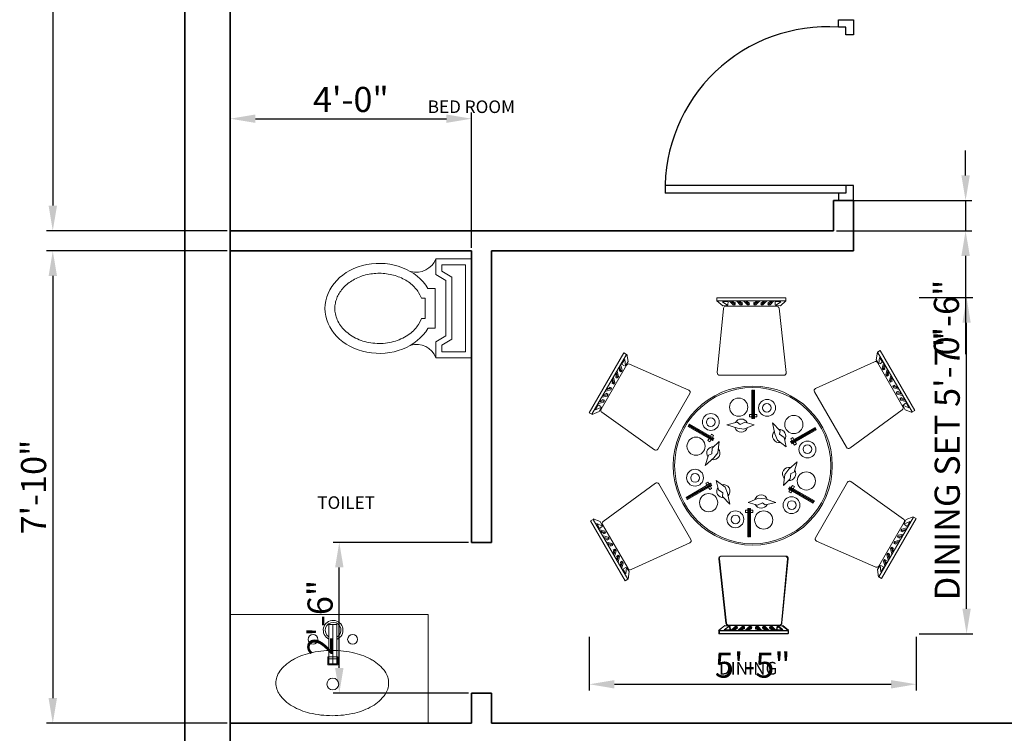
# Model space of a CAD drawing. Units: inches. Extents: x -24887 to 3061, y 1794 to 4919553.
# Tile 5 of 14: x 2132 to 2328, y 2076 to 2218. Entities that reach past the tile are written whole.
import ezdxf

# ---------------------------------------------------------------- set-up
doc = ezdxf.new("R2010")
doc.units = ezdxf.units.IN
for name, color, linetype, lineweight in [('A-ANNO-DIMS', 2, 'Continuous', 18), ('A-AREA-IDEN', 7, 'Continuous', 18), ('A-FLOR-FIXT', 9, 'Continuous', 18), ('A-FURN', 8, 'Continuous', 18), ('door', 4, 'Continuous', 25), ('wall', 7, 'Continuous', 35)]:
    doc.layers.add(name, color=color, linetype=linetype, lineweight=lineweight)
doc.styles.get("Standard").update_dxf_attribs({"font": 'arial.ttf'})
doc.dimstyles.new('ISO-25', dxfattribs={"dimtxt": 5, "dimasz": 5, "dimexe": 1.25, "dimexo": 0.625, "dimtad": 1, "dimdec": 1, "dimlunit": 3, "dimtxsty": 'Standard', "dimcen": 2.5, "dimadec": 0, "dimazin": 0, "dimtfac": 1, "dimtdec": 1, "dimtmove": 0, "dimatfit": 3, "dimfxl": 1, "dimarcsym": 0})

# ---------------------------------------------------------------- blocks, each defined once
blk = doc.blocks.new('A$C7C8779AE')
for p, q in [((0, 0.7405), (0, 0.5605)), ((0.5, 0.7405), (0, 0.7405)), ((0.47, 0.7105), (0.03, 0.7105)), ((0.03, 0.7105), (0.03, 0.5905)), ((0.47, 0.5905), (0.47, 0.7105)), ((0.5, 0.5605), (0.5, 0.7405)), ((0.093, 0.6405), (0.063, 0.5905)), ((0.11, 0.6105), (0.08, 0.5605)), ((0.093, 0.6405), (0.407, 0.6405)), ((0.11, 0.6105), (0.39, 0.6105)), ((0.42, 0.5605), (0.39, 0.6105)), ((0.437, 0.5905), (0.407, 0.6405)), ((0, 0.5605), (0.08, 0.5605)), ((0.03, 0.5905), (0.063, 0.5905)), ((0.1497, 0.557), (0.1497, 0.5203)), ((0.1497, 0.557), (0.3514, 0.557)), ((0.3514, 0.557), (0.3514, 0.5203)), ((0.42, 0.5605), (0.5, 0.5605)), ((0.437, 0.5905), (0.47, 0.5905)), ((0.1997, 0.507), (0.1997, 0.4879)), ((0.1997, 0.507), (0.3014, 0.507)), ((0.3014, 0.507), (0.3014, 0.4879))]:
    blk.add_line(p, q)
for centre, start, end in [((-0.0386, 0.4613), 344.642, 68.7339), ((0.5386, 0.4613), 111.2661, 195.358)]:
    blk.add_arc(centre, 0.1064, start, end)
blk.add_ellipse((0.2506, 0.2744), major_axis=(0, 0.2744), ratio=0.828948, start_param=0.459479, end_param=5.823706)
blk.add_open_spline([(0.1997, 0.4879), (0.1697, 0.474), (0.1642, 0.4702), (0.1512, 0.4602), (0.1438, 0.4535), (0.1298, 0.4388), (0.1233, 0.4306), (0.1111, 0.4131), (0.1055, 0.4037), (0.0956, 0.3838), (0.0912, 0.3733), (0.0838, 0.3516), (0.0808, 0.3403), (0.0762, 0.3172), (0.0746, 0.3055), (0.073, 0.2817), (0.0729, 0.2698), (0.0743, 0.246), (0.0758, 0.2342), (0.0801, 0.2111), (0.0831, 0.1998), (0.0903, 0.1779), (0.0945, 0.1673), (0.1043, 0.1473), (0.1098, 0.1378), (0.1218, 0.12), (0.1283, 0.1118), (0.1421, 0.0968), (0.1494, 0.09), (0.1646, 0.078), (0.1725, 0.0728), (0.1887, 0.064), (0.1969, 0.0603), (0.2137, 0.0547), (0.2222, 0.0527), (0.2392, 0.0502), (0.2478, 0.0498), (0.2664, 0.0505), (0.2764, 0.052), (0.2963, 0.0573), (0.3061, 0.061), (0.3253, 0.0707), (0.3346, 0.0766), (0.3525, 0.0906), (0.3611, 0.0987), (0.3771, 0.1169), (0.3845, 0.127), (0.3978, 0.1488), (0.4037, 0.1605), (0.4137, 0.1853), (0.4178, 0.1983), (0.424, 0.2251), (0.4261, 0.2389), (0.4282, 0.2668), (0.4283, 0.2809), (0.4262, 0.3088), (0.4241, 0.3226), (0.418, 0.3495), (0.414, 0.3625), (0.404, 0.3873), (0.3982, 0.3991), (0.385, 0.421), (0.3776, 0.4311), (0.3617, 0.4494), (0.3531, 0.4575), (0.3382, 0.4693), (0.3321, 0.4736), (0.3014, 0.4879)], degree=3, knots=[0.459479, 0.459479, 0.459479, 0.459479, 0.567422, 0.567422, 0.720865, 0.720865, 0.874307, 0.874307, 1.02775, 1.02775, 1.181192, 1.181192, 1.334635, 1.334635, 1.488077, 1.488077, 1.64152, 1.64152, 1.794963, 1.794963, 1.948405, 1.948405, 2.101848, 2.101848, 2.25529, 2.25529, 2.408733, 2.408733, 2.562175, 2.562175, 2.715618, 2.715618, 2.86906, 2.86906, 3.022503, 3.022503, 3.175946, 3.175946, 3.356457, 3.356457, 3.536968, 3.536968, 3.717479, 3.717479, 3.89799, 3.89799, 4.078501, 4.078501, 4.259012, 4.259012, 4.439523, 4.439523, 4.620035, 4.620035, 4.800546, 4.800546, 4.981057, 4.981057, 5.161568, 5.161568, 5.342079, 5.342079, 5.52259, 5.52259, 5.703101, 5.703101, 5.823706, 5.823706, 5.823706, 5.823706])
blk = doc.blocks.new('A$C45501D90')
for p, q in [((-242.2, 1133.5), (224, 1133.5)), ((-242.2, 1112.8), (-242.2, 1133.5)), ((224, 1133.5), (224, 1112.8)), ((224, 1112.8), (-242.2, 1112.8)), ((-242.2, 1111.2), (-202.3, 1079.2)), ((-203.9, 1106.4), (-165.6, 1108)), ((-168.8, 1080.8), (-203.9, 1106.4)), ((-202.3, 1079.2), (-168.8, 1080.8)), ((161.8, 1076.1), (-181.4, 1076.1)), ((-165.6, 1108), (-167.2, 1085.6)), ((-156, 1109.6), (-132, 1085.6)), ((-119.3, 1085.6), (-143.2, 1108)), ((-143.2, 1108), (-133.6, 1108)), ((-133.6, 1108), (-122.5, 1098.4)), ((-132, 1085.6), (-119.3, 1085.6)), ((-122.5, 1098.4), (-119.3, 1101.6)), ((-119.3, 1101.6), (-117.7, 1087.2)), ((-108.1, 1109.6), (-84.1, 1085.6)), ((-71.4, 1085.6), (-95.3, 1108)), ((-95.3, 1108), (-85.7, 1108)), ((-85.7, 1108), (-74.6, 1098.4)), ((-84.1, 1085.6), (-71.4, 1085.6)), ((-74.6, 1098.4), (-71.4, 1101.6)), ((-71.4, 1101.6), (-69.8, 1087.2)), ((-60.2, 1109.6), (-36.2, 1085.6)), ((-23.5, 1085.6), (-47.4, 1108)), ((-47.4, 1108), (-37.8, 1108)), ((-37.8, 1108), (-26.7, 1098.4)), ((-36.2, 1085.6), (-23.5, 1085.6)), ((-26.7, 1098.4), (-23.5, 1101.6)), ((-23.5, 1101.6), (-21.9, 1087.2)), ((8.5, 1101.6), (6.9, 1087.2)), ((8.5, 1085.6), (32.4, 1108)), ((11.6, 1098.4), (8.5, 1101.6)), ((21.2, 1085.6), (8.5, 1085.6)), ((22.8, 1108), (11.6, 1098.4)), ((45.2, 1109.6), (21.2, 1085.6)), ((32.4, 1108), (22.8, 1108)), ((56.3, 1101.6), (54.8, 1087.2)), ((56.3, 1085.6), (80.3, 1108)), ((59.5, 1098.4), (56.3, 1101.6)), ((69.1, 1085.6), (56.3, 1085.6)), ((70.7, 1108), (59.5, 1098.4)), ((93.1, 1109.6), (69.1, 1085.6)), ((80.3, 1108), (70.7, 1108)), ((104.2, 1101.6), (102.6, 1087.2)), ((104.2, 1085.6), (128.2, 1108)), ((107.4, 1098.4), (104.2, 1101.6)), ((117, 1085.6), (104.2, 1085.6)), ((118.6, 1108), (107.4, 1098.4)), ((141, 1109.6), (117, 1085.6)), ((128.2, 1108), (118.6, 1108)), ((188.9, 1106.4), (150.5, 1108)), ((150.5, 1108), (152.1, 1085.6)), ((153.7, 1080.8), (188.9, 1106.4)), ((187.3, 1079.2), (153.7, 1080.8)), ((224, 1112.8), (187.3, 1079.2)), ((-197.3, 1061.6), (-238.9, 627.6)), ((225.2, 627.8), (177.6, 1061.8)), ((-1102.7, 357), (-869.7, 760.7)), ((-851.7, 750.4), (-1084.8, 346.6)), ((-869.7, 760.7), (-851.7, 750.4)), ((-848.7, 752.3), (-841, 701.8)), ((841.2, 765.3), (833.5, 714.8)), ((842.6, 766.1), (860.5, 776.5)), ((1075.7, 362.4), (842.6, 766.1)), ((860.5, 776.5), (1093.6, 372.8)), ((-851, 678.1), (-1022.6, 380.9)), ((-895.4, 665), (-900.2, 656.7)), ((-888.1, 633.1), (-895.4, 665)), ((-890.4, 676.9), (-881.7, 644.2)), ((-863.7, 716.7), (-884.3, 684.4)), ((-884.3, 684.4), (-864.1, 674.6)), ((-859.2, 673.6), (-863.7, 716.7)), ((-841, 701.8), (-859.2, 673.6)), ((-431.1, 509), (-830.8, 684.8)), ((820.7, 701.7), (424.1, 520.7)), ((833.5, 714.8), (851.7, 686.6)), ((1012.8, 397.9), (841.2, 695.1)), ((851.7, 686.6), (856.2, 729.8)), ((856.2, 729.8), (876.7, 697.4)), ((876.7, 697.4), (856.6, 687.6)), ((882.9, 689.9), (874.2, 657.2)), ((880.6, 646.1), (887.9, 678)), ((887.9, 678), (892.7, 669.7)), ((892.7, 669.7), (890, 655.2)), ((-921.5, 600.8), (-925.8, 599.6)), ((-925.8, 599.6), (-914.2, 591)), ((-919.4, 623.5), (-924.2, 615.2)), ((-924.2, 615.2), (-921.5, 600.8)), ((-912, 591.6), (-919.4, 623.5)), ((-914.4, 635.4), (-905.6, 602.7)), ((-905.6, 602.7), (-912, 591.6)), ((-897.5, 642.2), (-901.9, 641.1)), ((-901.9, 641.1), (-890.2, 632.5)), ((-900.2, 656.7), (-897.5, 642.2)), ((-881.7, 644.2), (-888.1, 633.1)), ((-223, 610.1), (209.4, 610.1)), ((874.2, 657.2), (880.6, 646.1)), ((894.4, 654.1), (882.7, 645.5)), ((890, 655.2), (894.4, 654.1)), ((906.9, 648.4), (898.1, 615.7)), ((898.1, 615.7), (904.5, 604.6)), ((904.5, 604.6), (911.9, 636.5)), ((918.3, 612.6), (906.7, 604)), ((911.9, 636.5), (916.7, 628.2)), ((916.7, 628.2), (914, 613.8)), ((914, 613.8), (918.3, 612.6)), ((930.8, 606.9), (922.1, 574.2)), ((-945.4, 559.3), (-949.8, 558.1)), ((-949.8, 558.1), (-938.1, 549.6)), ((-943.3, 582), (-948.1, 573.8)), ((-948.1, 573.8), (-945.4, 559.3)), ((-936, 550.1), (-943.3, 582)), ((-938.3, 593.9), (-929.6, 561.2)), ((-929.6, 561.2), (-936, 550.1)), ((922.1, 574.2), (928.4, 563.1)), ((928.4, 563.1), (935.8, 595.1)), ((942.3, 571.1), (930.6, 562.6)), ((935.8, 595.1), (940.6, 586.8)), ((940.6, 586.8), (937.9, 572.3)), ((937.9, 572.3), (942.3, 571.1)), ((950.8, 524.4), (944.4, 535.5)), ((944.4, 535.5), (975.7, 525.9)), ((958.2, 543.5), (945, 537.7)), ((957.1, 539.1), (958.2, 543.5)), ((970.9, 534.2), (957.1, 539.1)), ((975.7, 525.9), (970.9, 534.2)), ((-1015, 461.2), (-982.3, 469.9)), ((-975.9, 481), (-1007.2, 471.4)), ((-1007.2, 471.4), (-1002.4, 479.7)), ((-1002.4, 479.7), (-988.5, 484.6)), ((-991, 502.7), (-958.3, 511.4)), ((-988.5, 484.6), (-989.7, 489)), ((-989.7, 489), (-976.5, 483.2)), ((-951.9, 522.5), (-983.2, 512.9)), ((-983.2, 512.9), (-978.5, 521.2)), ((-982.3, 469.9), (-975.9, 481)), ((-978.5, 521.2), (-964.6, 526.1)), ((-964.6, 526.1), (-965.7, 530.5)), ((-965.7, 530.5), (-952.5, 524.7)), ((-958.3, 511.4), (-951.9, 522.5)), ((-639.9, 111.9), (-423.7, 486.4)), ((-5.6, 508.7, 90.8), (0.4, 508.7, 90.8)), ((-5.6, 317.7, 90.8), (-5.6, 508.7, 90.8)), ((0.4, 508.7, 90.8), (0.4, 317.7, 90.8)), ((5.8, 317.7, 90.8), (5.8, 508.7, 90.8)), ((5.8, 508.7, 90.8), (11.8, 508.7, 90.8)), ((11.8, 508.7, 90.8), (11.8, 317.7, 90.8)), ((416.9, 498.2), (633.1, 123.7)), ((983.5, 515.7), (950.8, 524.4)), ((968.4, 494), (999.7, 484.4)), ((974.7, 483), (968.4, 494)), ((982.2, 502), (968.9, 496.2)), ((1007.4, 474.2), (974.7, 483)), ((981, 497.6), (982.2, 502)), ((994.9, 492.7), (981, 497.6)), ((999.7, 484.4), (994.9, 492.7)), ((-1060.1, 376.6), (-1042.3, 410.6)), ((-1042.3, 410.6), (-1023.8, 398.1)), ((-1038.9, 419.7), (-1006.2, 428.5)), ((-999.8, 439.5), (-1031.1, 430)), ((-1031.1, 430), (-1026.3, 438.3)), ((-1026.3, 438.3), (-1012.5, 443.1)), ((-1012.5, 443.1), (-1013.6, 447.5)), ((-1013.6, 447.5), (-1000.4, 441.7)), ((-1006.2, 428.5), (-999.8, 439.5)), ((998.7, 441.5), (992.3, 452.5)), ((992.3, 452.5), (1023.6, 443)), ((1006.1, 460.5), (992.9, 454.7)), ((1031.4, 432.7), (998.7, 441.5)), ((1005, 456.2), (1006.1, 460.5)), ((1018.8, 451.3), (1005, 456.2)), ((1028.3, 377.5), (1012.9, 407.3)), ((1012.9, 407.3), (1052.6, 389.6)), ((1034.8, 423.6), (1016.3, 411.1)), ((1023.6, 443), (1018.8, 451.3)), ((1052.6, 389.6), (1034.8, 423.6)), ((-1084.8, 346.6), (-1102.7, 357)), ((-1083.4, 345.8), (-1035.8, 364.4)), ((-1020.4, 394.3), (-1060.1, 376.6)), ((-1035.8, 364.4), (-1020.4, 394.3)), ((-1018, 360), (-663, 106.9)), ((-22.3, 329.1, 90.8), (-22.3, 344.6, 90.8)), ((-22.3, 344.6, 90.8), (-5.6, 344.6, 90.8)), ((0.4, 344.6, 90.8), (5.8, 344.6, 90.8)), ((11.8, 344.6, 90.8), (27.3, 344.6, 90.8)), ((27.3, 344.6, 90.8), (27.3, 329.1, 90.8)), ((656.3, 118.9), (1008.4, 377.1)), ((1075.9, 358.8), (1028.3, 377.5)), ((1093.6, 372.8), (1075.7, 362.4)), ((-436.3, 265.3, 90.8), (-433.3, 270.5, 90.8)), ((-433.3, 270.5, 90.8), (-267.9, 175, 90.8)), ((-430.6, 275.2, 90.8), (-427.6, 280.3, 90.8)), ((-265.2, 179.7, 90.8), (-430.6, 275.2, 90.8)), ((-427.6, 280.3, 90.8), (-262.3, 184.9, 90.8)), ((-175.3, 276.1, 90.8), (-104.8, 293.2, 90.8)), ((-103.3, 252.4, 90.8), (-175.3, 276.1, 90.8)), ((-104.8, 293.2, 90.8), (-85.5, 278.4, 90.8)), ((-85.5, 278.4, 90.8), (-52.1, 293.9, 90.8)), ((9.5, 276.1, 90.8), (-59.5, 246.5, 90.8)), ((-52.1, 293.9, 90.8), (9.5, 276.1, 90.8)), ((-5.6, 329.1, 90.8), (-22.3, 329.1, 90.8)), ((0.4, 317.7, 90.8), (-5.6, 317.7, 90.8)), ((5.8, 329.1, 90.8), (0.4, 329.1, 90.8)), ((11.8, 317.7, 90.8), (5.8, 317.7, 90.8)), ((27.3, 329.1, 90.8), (11.8, 329.1, 90.8)), ((134.3, 288, 90.8), (184.3, 235.5, 90.8)), ((149.7, 213.9, 90.8), (134.3, 288, 90.8)), ((-270.9, 169.9, 90.8), (-436.3, 265.3, 90.8)), ((-285.5, 198.3, 90.8), (-277.8, 211.7, 90.8)), ((-277.8, 211.7, 90.8), (-264.3, 204, 90.8)), ((-264.3, 204, 90.8), (-272.1, 190.5, 90.8)), ((-59.5, 246.5, 90.8), (-103.3, 252.4, 90.8)), ((166.5, 173, 90.8), (149.7, 213.9, 90.8)), ((184.3, 235.5, 90.8), (181.1, 211.4, 90.8)), ((181.1, 211.4, 90.8), (211.3, 190.3, 90.8)), ((255.2, 161.9, 90.8), (420.6, 257.3, 90.8)), ((423.5, 252.2, 90.8), (258.2, 156.7, 90.8)), ((260.9, 152, 90.8), (426.2, 247.5, 90.8)), ((429.2, 242.3, 90.8), (263.8, 146.9, 90.8)), ((420.6, 257.3, 90.8), (423.5, 252.2, 90.8)), ((426.2, 247.5, 90.8), (429.2, 242.3, 90.8)), ((-302.5, 168.8, 90.8), (-294.2, 183.3, 90.8)), ((-289.1, 161.1, 90.8), (-302.5, 168.8, 90.8)), ((-291.2, 188.5, 90.8), (-288.5, 193.1, 90.8)), ((-280.7, 175.5, 90.8), (-289.1, 161.1, 90.8)), ((-275.1, 185.4, 90.8), (-277.8, 180.7, 90.8)), ((-273.6, 117.6, 90.8), (-227.4, 162.1, 90.8)), ((-267.9, 175, 90.8), (-270.9, 169.9, 90.8)), ((-262.3, 184.9, 90.8), (-265.2, 179.7, 90.8)), ((-227.4, 162.1, 90.8), (-236.2, 87.5, 90.8)), ((226.7, 128.1, 90.8), (166.5, 173, 90.8)), ((211.3, 190.3, 90.8), (226.7, 128.1, 90.8)), ((258.2, 156.7, 90.8), (255.2, 161.9, 90.8)), ((256.6, 182, 90.8), (270.1, 189.8, 90.8)), ((265, 167.5, 90.8), (256.6, 182, 90.8)), ((263.8, 146.9, 90.8), (260.9, 152, 90.8)), ((270.7, 157.7, 90.8), (268, 162.4, 90.8)), ((270.1, 189.8, 90.8), (278.4, 175.3, 90.8)), ((281.4, 139.1, 90.8), (273.7, 152.5, 90.8)), ((281.4, 170.1, 90.8), (284.1, 165.5, 90.8)), ((294.9, 146.8, 90.8), (281.4, 139.1, 90.8)), ((287.1, 160.3, 90.8), (294.9, 146.8, 90.8)), ((-319.8, 2.1, 90.8), (-299.3, 71.7, 90.8)), ((-299.3, 71.7, 90.8), (-276.8, 80.9, 90.8)), ((-276.8, 80.9, 90.8), (-273.6, 117.6, 90.8)), ((-236.2, 87.5, 90.8), (-263.2, 52.5, 90.8)), ((-263.2, 52.5, 90.8), (-319.8, 2.1, 90.8)), ((242.9, -24.6, 90.8), (299.4, 25.9, 90.8)), ((299.4, 25.9, 90.8), (278.9, -43.7, 90.8)), ((207, -134.1, 90.8), (215.8, -59.5, 90.8)), ((215.8, -59.5, 90.8), (242.9, -24.6, 90.8)), ((256.4, -53, 90.8), (253.2, -89.7, 90.8)), ((278.9, -43.7, 90.8), (256.4, -53, 90.8)), ((-656.3, -118.9), (-1008.4, -377.1)), ((-416.9, -498.2), (-633.1, -123.7)), ((-449.6, -214.4, 90.8), (-284.2, -118.9, 90.8)), ((-281.2, -124.1, 90.8), (-446.6, -219.5, 90.8)), ((-443.9, -224.2, 90.8), (-278.5, -128.7, 90.8)), ((-315.2, -118.9, 90.8), (-301.8, -111.1, 90.8)), ((-307.5, -132.3, 90.8), (-315.2, -118.9, 90.8)), ((-301.8, -111.1, 90.8), (-294, -124.6, 90.8)), ((-291, -129.7, 90.8), (-288.3, -134.4, 90.8)), ((-284.2, -118.9, 90.8), (-281.2, -124.1, 90.8)), ((-278.5, -128.7, 90.8), (-275.5, -133.9, 90.8)), ((-247, -100.1, 90.8), (-186.8, -145, 90.8)), ((-231.7, -162.3, 90.8), (-247, -100.1, 90.8)), ((253.2, -89.7, 90.8), (207, -134.1, 90.8)), ((639.9, -111.9), (423.7, -486.4)), ((1018, -360), (663, -106.9)), ((-275.5, -133.9, 90.8), (-440.9, -229.4, 90.8)), ((-301.8, -142.1, 90.8), (-304.5, -137.5, 90.8)), ((-290.4, -161.8, 90.8), (-298.8, -147.3, 90.8)), ((-277, -154, 90.8), (-290.4, -161.8, 90.8)), ((-285.4, -139.5, 90.8), (-277, -154, 90.8)), ((-201.5, -183.4, 90.8), (-231.7, -162.3, 90.8)), ((-204.7, -207.6, 90.8), (-201.5, -183.4, 90.8)), ((-186.8, -145, 90.8), (-170.1, -185.9, 90.8)), ((-170.1, -185.9, 90.8), (-154.7, -260.1, 90.8)), ((241.9, -156.9, 90.8), (244.9, -151.7, 90.8)), ((407.3, -252.4, 90.8), (241.9, -156.9, 90.8)), ((244, -176, 90.8), (251.7, -162.5, 90.8)), ((257.4, -183.7, 90.8), (244, -176, 90.8)), ((244.9, -151.7, 90.8), (410.3, -247.2, 90.8)), ((247.6, -147.1, 90.8), (250.6, -141.9, 90.8)), ((413, -242.5, 90.8), (247.6, -147.1, 90.8)), ((250.6, -141.9, 90.8), (415.9, -237.4, 90.8)), ((254.7, -157.4, 90.8), (257.4, -152.7, 90.8)), ((265.2, -170.3, 90.8), (257.4, -183.7, 90.8)), ((260.4, -147.6, 90.8), (268.7, -133.1, 90.8)), ((270.8, -160.5, 90.8), (268.1, -165.1, 90.8)), ((268.7, -133.1, 90.8), (282.2, -140.8, 90.8)), ((282.2, -140.8, 90.8), (273.8, -155.3, 90.8)), ((-446.6, -219.5, 90.8), (-449.6, -214.4, 90.8)), ((-440.9, -229.4, 90.8), (-443.9, -224.2, 90.8)), ((-154.7, -260.1, 90.8), (-204.7, -207.6, 90.8)), ((-29.8, -248.2, 90.8), (39.2, -218.5, 90.8)), ((31.8, -266, 90.8), (-29.8, -248.2, 90.8)), ((65.2, -250.4, 90.8), (31.8, -266, 90.8)), ((39.2, -218.5, 90.8), (83, -224.4, 90.8)), ((84.4, -265.2, 90.8), (65.2, -250.4, 90.8)), ((83, -224.4, 90.8), (154.9, -248.2, 90.8)), ((154.9, -248.2, 90.8), (84.4, -265.2, 90.8)), ((410.3, -247.2, 90.8), (407.3, -252.4, 90.8)), ((415.9, -237.4, 90.8), (413, -242.5, 90.8)), ((-47.6, -316.6, 90.8), (-47.6, -301.1, 90.8)), ((-47.6, -301.1, 90.8), (-32.1, -301.1, 90.8)), ((-32.1, -316.6, 90.8), (-47.6, -316.6, 90.8)), ((-32.1, -480.7, 90.8), (-32.1, -289.8, 90.8)), ((-32.1, -289.8, 90.8), (-26.1, -289.8, 90.8)), ((-26.1, -289.8, 90.8), (-26.1, -480.7, 90.8)), ((-26.1, -301.1, 90.8), (-20.8, -301.1, 90.8)), ((-20.8, -316.6, 90.8), (-26.1, -316.6, 90.8)), ((-20.8, -480.7, 90.8), (-20.8, -289.8, 90.8)), ((-20.8, -289.8, 90.8), (-14.8, -289.8, 90.8)), ((-14.8, -289.8, 90.8), (-14.8, -480.7, 90.8)), ((-14.8, -301.1, 90.8), (1.9, -301.1, 90.8)), ((1.9, -316.6, 90.8), (-14.8, -316.6, 90.8)), ((1.9, -301.1, 90.8), (1.9, -316.6, 90.8)), ((-1093.6, -372.8), (-1075.7, -362.4)), ((-860.5, -776.5), (-1093.6, -372.8)), ((-1075.9, -358.8), (-1028.3, -377.5)), ((-1075.7, -362.4), (-842.6, -766.1)), ((-1052.6, -389.6), (-1034.8, -423.6)), ((-1012.9, -407.3), (-1052.6, -389.6)), ((-1028.3, -377.5), (-1012.9, -407.3)), ((-1012.8, -397.9), (-841.2, -695.1)), ((851, -678.1), (1022.6, -380.9)), ((851.7, -750.4), (1084.8, -346.6)), ((1102.7, -357), (869.7, -760.7)), ((1035.8, -364.4), (1020.4, -394.3)), ((1020.4, -394.3), (1060.1, -376.6)), ((1042.3, -410.6), (1023.8, -398.1)), ((1083.4, -345.8), (1035.8, -364.4)), ((1060.1, -376.6), (1042.3, -410.6)), ((1084.8, -346.6), (1102.7, -357)), ((-1034.8, -423.6), (-1016.3, -411.1)), ((-1031.4, -432.7), (-998.7, -441.5)), ((-1023.6, -443), (-1018.8, -451.3)), ((-992.3, -452.5), (-1023.6, -443)), ((-1018.8, -451.3), (-1005, -456.2)), ((-1006.1, -460.5), (-992.9, -454.7)), ((-1005, -456.2), (-1006.1, -460.5)), ((-998.7, -441.5), (-992.3, -452.5)), ((1015, -461.2), (982.3, -469.9)), ((1006.2, -428.5), (999.8, -439.5)), ((999.8, -439.5), (1031.1, -430)), ((1013.6, -447.5), (1000.4, -441.7)), ((1038.9, -419.7), (1006.2, -428.5)), ((1026.3, -438.3), (1012.5, -443.1)), ((1012.5, -443.1), (1013.6, -447.5)), ((1031.1, -430), (1026.3, -438.3)), ((-1007.4, -474.2), (-974.7, -483)), ((-968.4, -494), (-999.7, -484.4)), ((-999.7, -484.4), (-994.9, -492.7)), ((-994.9, -492.7), (-981, -497.6)), ((-983.5, -515.7), (-950.8, -524.4)), ((-982.2, -502), (-968.9, -496.2)), ((-981, -497.6), (-982.2, -502)), ((-944.4, -535.5), (-975.7, -525.9)), ((-975.7, -525.9), (-970.9, -534.2)), ((-974.7, -483), (-968.4, -494)), ((-950.8, -524.4), (-944.4, -535.5)), ((-820.7, -701.7), (-424.1, -520.7)), ((-26.1, -480.7, 90.8), (-32.1, -480.7, 90.8)), ((-14.8, -480.7, 90.8), (-20.8, -480.7, 90.8)), ((431.1, -509), (830.8, -684.8)), ((958.3, -511.4), (951.9, -522.5)), ((951.9, -522.5), (983.2, -512.9)), ((965.7, -530.5), (952.5, -524.7)), ((991, -502.7), (958.3, -511.4)), ((978.5, -521.2), (964.6, -526.1)), ((964.6, -526.1), (965.7, -530.5)), ((982.3, -469.9), (975.9, -481)), ((975.9, -481), (1007.2, -471.4)), ((989.7, -489), (976.5, -483.2)), ((983.2, -512.9), (978.5, -521.2)), ((1002.4, -479.7), (988.5, -484.6)), ((988.5, -484.6), (989.7, -489)), ((1007.2, -471.4), (1002.4, -479.7)), ((-970.9, -534.2), (-957.1, -539.1)), ((-958.2, -543.5), (-945, -537.7)), ((-957.1, -539.1), (-958.2, -543.5)), ((-942.3, -571.1), (-930.6, -562.6)), ((-937.9, -572.3), (-942.3, -571.1)), ((-940.6, -586.8), (-937.9, -572.3)), ((-935.8, -595.1), (-940.6, -586.8)), ((-928.4, -563.1), (-935.8, -595.1)), ((-930.8, -606.9), (-922.1, -574.2)), ((-922.1, -574.2), (-928.4, -563.1)), ((905.6, -602.7), (912, -591.6)), ((912, -591.6), (919.4, -623.5)), ((925.8, -599.6), (914.2, -591)), ((929.6, -561.2), (936, -550.1)), ((938.3, -593.9), (929.6, -561.2)), ((936, -550.1), (943.3, -582)), ((949.8, -558.1), (938.1, -549.6)), ((943.3, -582), (948.1, -573.8)), ((945.4, -559.3), (949.8, -558.1)), ((948.1, -573.8), (945.4, -559.3)), ((-918.3, -612.6), (-906.7, -604)), ((-914, -613.8), (-918.3, -612.6)), ((-916.7, -628.2), (-914, -613.8)), ((-911.9, -636.5), (-916.7, -628.2)), ((-904.5, -604.6), (-911.9, -636.5)), ((-906.9, -648.4), (-898.1, -615.7)), ((-898.1, -615.7), (-904.5, -604.6)), ((-894.4, -654.1), (-882.7, -645.5)), ((-890, -655.2), (-894.4, -654.1)), ((-892.7, -669.7), (-890, -655.2)), ((-880.6, -646.1), (-887.9, -678)), ((-882.9, -689.9), (-874.2, -657.2)), ((-874.2, -657.2), (-880.6, -646.1)), ((-229.3, -629.3), (-181.8, -1063.3)), ((-225.2, -627.8), (-177.6, -1061.8)), ((218.9, -611.6), (-213.5, -611.6)), ((223, -610.1), (-209.4, -610.1)), ((193.2, -1063.1), (234.8, -629.1)), ((197.3, -1061.6), (238.9, -627.6)), ((881.7, -644.2), (888.1, -633.1)), ((890.4, -676.9), (881.7, -644.2)), ((888.1, -633.1), (895.4, -665)), ((901.9, -641.1), (890.2, -632.5)), ((895.4, -665), (900.2, -656.7)), ((897.5, -642.2), (901.9, -641.1)), ((900.2, -656.7), (897.5, -642.2)), ((914.4, -635.4), (905.6, -602.7)), ((919.4, -623.5), (924.2, -615.2)), ((921.5, -600.8), (925.8, -599.6)), ((924.2, -615.2), (921.5, -600.8)), ((-887.9, -678), (-892.7, -669.7)), ((-876.7, -697.4), (-856.6, -687.6)), ((-856.2, -729.8), (-876.7, -697.4)), ((-851.7, -686.6), (-856.2, -729.8)), ((-833.5, -714.8), (-851.7, -686.6)), ((-841.2, -765.3), (-833.5, -714.8)), ((841, -701.8), (859.2, -673.6)), ((848.7, -752.3), (841, -701.8)), ((859.2, -673.6), (863.7, -716.7)), ((863.7, -716.7), (884.3, -684.4)), ((884.3, -684.4), (864.1, -674.6)), ((-842.6, -766.1), (-860.5, -776.5)), ((869.7, -760.7), (851.7, -750.4)), ((-231.3, -1112.7), (-191.4, -1080.8)), ((-228.1, -1114.3), (238.1, -1114.3)), ((-228.1, -1135), (-228.1, -1114.3)), ((-227.2, -1111.2), (-187.3, -1079.2)), ((-224, -1112.8), (242.2, -1112.8)), ((-224, -1133.5), (-224, -1112.8)), ((-157.9, -1082.4), (-193, -1107.9)), ((-193, -1107.9), (-154.7, -1109.5)), ((-191.4, -1080.8), (-157.9, -1082.4)), ((-153.7, -1080.8), (-188.9, -1106.4)), ((-188.9, -1106.4), (-150.5, -1108)), ((-187.3, -1079.2), (-153.7, -1080.8)), ((-165.9, -1077.6), (177.3, -1077.6)), ((-161.8, -1076.1), (181.4, -1076.1)), ((-154.7, -1109.5), (-156.3, -1087.1)), ((-150.5, -1108), (-152.1, -1085.6)), ((-145.1, -1111.1), (-121.1, -1087.1)), ((-141, -1109.6), (-117, -1085.6)), ((-108.4, -1087.1), (-132.3, -1109.5)), ((-132.3, -1109.5), (-122.7, -1109.5)), ((-104.2, -1085.6), (-128.2, -1108)), ((-128.2, -1108), (-118.6, -1108)), ((-122.7, -1109.5), (-111.6, -1099.9)), ((-121.1, -1087.1), (-108.4, -1087.1)), ((-118.6, -1108), (-107.4, -1098.4)), ((-117, -1085.6), (-104.2, -1085.6)), ((-111.6, -1099.9), (-108.4, -1103.1)), ((-108.4, -1103.1), (-106.8, -1088.7)), ((-107.4, -1098.4), (-104.2, -1101.6)), ((-104.2, -1101.6), (-102.6, -1087.2)), ((-97.2, -1111.1), (-73.2, -1087.1)), ((-93.1, -1109.6), (-69.1, -1085.6)), ((-60.5, -1087.1), (-84.4, -1109.5)), ((-84.4, -1109.5), (-74.8, -1109.5)), ((-56.3, -1085.6), (-80.3, -1108)), ((-80.3, -1108), (-70.7, -1108)), ((-74.8, -1109.5), (-63.7, -1099.9)), ((-73.2, -1087.1), (-60.5, -1087.1)), ((-70.7, -1108), (-59.5, -1098.4)), ((-69.1, -1085.6), (-56.3, -1085.6)), ((-63.7, -1099.9), (-60.5, -1103.1)), ((-60.5, -1103.1), (-58.9, -1088.7)), ((-59.5, -1098.4), (-56.3, -1101.6)), ((-56.3, -1101.6), (-54.8, -1087.2)), ((-49.3, -1111.1), (-25.3, -1087.1)), ((-45.2, -1109.6), (-21.2, -1085.6)), ((-12.6, -1087.1), (-36.5, -1109.5)), ((-36.5, -1109.5), (-26.9, -1109.5)), ((-8.5, -1085.6), (-32.4, -1108)), ((-32.4, -1108), (-22.8, -1108)), ((-26.9, -1109.5), (-15.8, -1099.9)), ((-25.3, -1087.1), (-12.6, -1087.1)), ((-22.8, -1108), (-11.6, -1098.4)), ((-21.2, -1085.6), (-8.5, -1085.6)), ((-15.8, -1099.9), (-12.6, -1103.1)), ((-12.6, -1103.1), (-11, -1088.7)), ((-11.6, -1098.4), (-8.5, -1101.6)), ((-8.5, -1101.6), (-6.9, -1087.2)), ((19.4, -1103.1), (17.8, -1088.7)), ((19.4, -1087.1), (43.3, -1109.5)), ((32.1, -1087.1), (19.4, -1087.1)), ((22.6, -1099.9), (19.4, -1103.1)), ((23.5, -1101.6), (21.9, -1087.2)), ((33.7, -1109.5), (22.6, -1099.9)), ((23.5, -1085.6), (47.4, -1108)), ((36.2, -1085.6), (23.5, -1085.6)), ((26.7, -1098.4), (23.5, -1101.6)), ((37.8, -1108), (26.7, -1098.4)), ((56.1, -1111.1), (32.1, -1087.1)), ((43.3, -1109.5), (33.7, -1109.5)), ((60.2, -1109.6), (36.2, -1085.6)), ((47.4, -1108), (37.8, -1108)), ((67.3, -1103.1), (65.7, -1088.7)), ((67.3, -1087.1), (91.2, -1109.5)), ((80, -1087.1), (67.3, -1087.1)), ((70.4, -1099.9), (67.3, -1103.1)), ((71.4, -1101.6), (69.8, -1087.2)), ((81.6, -1109.5), (70.4, -1099.9)), ((71.4, -1085.6), (95.3, -1108)), ((84.1, -1085.6), (71.4, -1085.6)), ((74.6, -1098.4), (71.4, -1101.6)), ((85.7, -1108), (74.6, -1098.4)), ((104, -1111.1), (80, -1087.1)), ((91.2, -1109.5), (81.6, -1109.5)), ((108.1, -1109.6), (84.1, -1085.6)), ((95.3, -1108), (85.7, -1108)), ((115.1, -1103.1), (113.6, -1088.7)), ((115.1, -1087.1), (139.1, -1109.5)), ((127.9, -1087.1), (115.1, -1087.1)), ((118.3, -1099.9), (115.1, -1103.1)), ((119.3, -1101.6), (117.7, -1087.2)), ((129.5, -1109.5), (118.3, -1099.9)), ((119.3, -1085.6), (143.2, -1108)), ((132, -1085.6), (119.3, -1085.6)), ((122.5, -1098.4), (119.3, -1101.6)), ((133.6, -1108), (122.5, -1098.4)), ((151.9, -1111.1), (127.9, -1087.1)), ((139.1, -1109.5), (129.5, -1109.5)), ((156, -1109.6), (132, -1085.6)), ((143.2, -1108), (133.6, -1108)), ((161.4, -1109.5), (163, -1087.1)), ((199.8, -1107.9), (161.4, -1109.5)), ((198.2, -1080.8), (164.6, -1082.4)), ((164.6, -1082.4), (199.8, -1107.9)), ((165.6, -1108), (167.2, -1085.6)), ((203.9, -1106.4), (165.6, -1108)), ((202.3, -1079.2), (168.8, -1080.8)), ((168.8, -1080.8), (203.9, -1106.4)), ((238.1, -1112.7), (198.2, -1080.8)), ((242.2, -1111.2), (202.3, -1079.2)), ((238.1, -1114.3), (238.1, -1135)), ((242.2, -1112.8), (242.2, -1133.5)), ((238.1, -1135), (-228.1, -1135)), ((242.2, -1133.5), (-224, -1133.5))]:
    blk.add_line(p, q)
for centre, radius in [((0, 0), 537), ((0, 0), 527), ((-94.8, 394.7, 90.8), 61.3), ((96.9, 390, 90.8), 56.9), ((95.5, 390.7, 90.8), 29.4), ((-282.3, 294.7, 90.8), 56.9), ((277.2, 277.6, 90.8), 61.3), ((-283.5, 293.9, 90.8), 29.4), ((-382.1, 131.1, 90.8), 61.3), ((369, 109.3, 90.8), 56.9), ((368.9, 110.8, 90.8), 29.4), ((-389.3, -81.3, 90.8), 56.9), ((-389.2, -82.8, 90.8), 29.4), ((361.8, -103.1, 90.8), 61.3), ((-297.5, -249.6, 90.8), 61.3), ((261.9, -266.7, 90.8), 56.9), ((263.2, -265.9, 90.8), 29.4), ((-117.2, -362, 90.8), 56.9), ((74.4, -366.7, 90.8), 61.3), ((-115.9, -362.7, 90.8), 29.4)]:
    blk.add_circle(centre, radius)
for centre, radius, start, end in [((-181.4, 1060.1), 16, 90, 174.51988), ((161.8, 1060.1), 16, 6.25717, 90), ((-837.2, 670.1), 16, 66.25717, 150), ((827.4, 687.1), 16, 30, 114.51988), ((-223, 626.1), 16, 174.51988, 270), ((209.4, 626.1), 16, 270, 6.25717), ((-437.5, 494.4), 16, 330, 66.25717), ((430.7, 506.2), 16, 114.51988, 210), ((-1008.8, 373), 16, 150, 234.51988), ((999, 389.9), 16, 306.25717, 30), ((-77.3, 270.2, 90.8), 44.6, 25.85584, 153.33587), ((-77.3, 270.2, 90.8), 44.6, 195.93383, 342.9389), ((178.1, 200.3, 90.8), 44.6, 135.93383, 282.9389), ((178.1, 200.3, 90.8), 44.6, 325.85584, 93.33587), ((-653.7, 119.9), 16, 234.51988, 330), ((-265.7, 83.9, 90.8), 44.6, 85.85584, 213.33587), ((-265.7, 83.9, 90.8), 44.6, 255.93383, 42.9389), ((646.9, 131.7), 16, 210, 306.25717), ((245.3, -55.9, 90.8), 44.6, 75.93383, 222.9389), ((245.3, -55.9, 90.8), 44.6, 265.85584, 33.33587), ((-646.9, -131.7), 16, 30, 126.25717), ((-198.5, -172.3, 90.8), 44.6, 315.93383, 102.9389), ((653.7, -119.9), 16, 54.51988, 150), ((-198.5, -172.3, 90.8), 44.6, 145.85584, 273.33587), ((57, -242.2, 90.8), 44.6, 15.93383, 162.9389), ((57, -242.2, 90.8), 44.6, 205.85584, 333.33587), ((-999, -389.9), 16, 126.25717, 210), ((1008.8, -373), 16, 330, 54.51988), ((-430.7, -506.2), 16, 294.51988, 30), ((437.5, -494.4), 16, 150, 246.25717), ((-213.5, -627.6), 16, 90, 186.25717), ((-209.4, -626.1), 16, 90, 186.25717), ((218.9, -627.6), 16, 354.51988, 90), ((223, -626.1), 16, 354.51988, 90), ((-827.4, -687.1), 16, 210, 294.51988), ((837.2, -670.1), 16, 246.25717, 330), ((-161.8, -1060.1), 16, 186.25717, 270), ((181.4, -1060.1), 16, 270, 354.51988), ((-165.9, -1061.6), 16, 186.25717, 270), ((177.3, -1061.6), 16, 270, 354.51988)]:
    blk.add_arc(centre, radius, start, end)
blk = doc.blocks.new('A$C50A015BB')
for p, q in [((0, 0.55), (1, 0.55)), ((0, 0.55), (0, 0)), ((1, 0.55), (1, 0)), ((0.4985, 0.5), (0.5385, 0.5)), ((0.4985, 0.5), (0.4985, 0.3)), ((0.5185, 0.5), (0.5185, 0.3)), ((0.5385, 0.5), (0.5385, 0.3)), ((0.4935, 0.335), (0.4935, 0.295)), ((0.4935, 0.335), (0.5435, 0.335)), ((0.4985, 0.325), (0.5385, 0.325)), ((0.4985, 0.3), (0.5385, 0.3)), ((0.5435, 0.335), (0.5435, 0.295)), ((0.4935, 0.295), (0.5435, 0.295)), ((0, 0), (1, 0)), ((0, 0), (1, 0))]:
    blk.add_line(p, q)
for centre, radius in [((0.4185, 0.424), 0.025), ((0.6185, 0.424), 0.025), ((0.5185, 0.1981), 0.0298)]:
    blk.add_circle(centre, radius)
for centre, radius, start, end in [((0.5201, 0.4703), 0.0497, 291.7425, 244.2331), ((0.5201, 0.4703), 0.0397, 297.632, 237.0256), ((0.4772, 0.0383), 0.3252, 103.4853, 120.0686), ((0.5157, -0.1225), 0.4906, 90, 103.4853), ((0.5157, -0.1225), 0.4906, 76.5147, 90), ((0.5543, 0.0383), 0.3252, 59.9314, 76.5147), ((0.4185, 0.1397), 0.2081, 120.0686, 144.4178), ((0.613, 0.1397), 0.2081, 35.5822, 59.9314), ((0.3299, 0.2031), 0.0991, 144.4178, 180), ((0.7016, 0.2031), 0.0991, 0, 35.5822), ((0.3299, 0.2031), 0.0991, 180, 215.5822), ((0.7016, 0.2031), 0.0991, 324.4178, 0), ((0.4185, 0.2665), 0.2081, 215.5822, 239.9314), ((0.613, 0.2665), 0.2081, 300.0686, 324.4178), ((0.4772, 0.3679), 0.3252, 239.9314, 256.5147), ((0.5157, 0.5288), 0.4906, 256.5147, 270), ((0.5157, 0.5288), 0.4906, 270, 283.4853), ((0.5543, 0.3679), 0.3252, 283.4853, 300.0686)]:
    blk.add_arc(centre, radius, start, end)
blk = doc.blocks.new('DOOR-SINGLE-36IN')
for p, q in [((34.5, 36), (37.5, 36)), ((34.5, 34.5), (34.5, 36)), ((37.5, 36), (37.5, 33)), ((36, 34.5), (34.5, 34.5)), ((36, 33), (36, 34.5)), ((37.5, 33), (36, 33)), ((36, 3), (0, 3)), ((37.5, 3), (36, 3)), ((36, 3), (36, 1.5)), ((37.5, 0), (37.5, 3)), ((36, 1.5), (0, 1.5)), ((36, 1.5), (34.5, 1.5)), ((34.5, 1.5), (34.5, 0)), ((34.5, 0), (37.5, 0))]:
    blk.add_line(p, q)
blk.add_arc((32.32, 2.25), 32.32, 86.1244, 181.3295)
blk = doc.blocks.new('*D52')
at = {"layer": 'A-ANNO-DIMS', "color": 0, "lineweight": -2, "transparency": 16777216}
for p, q in [((2311.01, 2162.63), (2321.67, 2162.63)), ((2320.42, 2100.73), (2320.42, 2157.63)), ((2311.01, 2095.73), (2321.67, 2095.73))]:
    blk.add_line(p, q, dxfattribs=at)
at = {"layer": 'A-ANNO-DIMS', "color": 0, "transparency": 16777216}
for points in [[(2319.59, 2157.63), (2321.25, 2157.63), (2320.42, 2162.63)], [(2319.59, 2100.73), (2321.25, 2100.73), (2320.42, 2095.73)]]:
    blk.add_solid(points, dxfattribs=at)
at = {"layer": 'Defpoints', "color": 0, "transparency": 16777216}
for p in [(2310.39, 2162.63), (2320.42, 2162.63), (2310.39, 2095.73)]:
    blk.add_point(p, dxfattribs=at)
at = {"layer": 'A-ANNO-DIMS', "color": 0, "transparency": 16777216, "insert": (2317.21, 2129.18), "char_height": 5, "attachment_point": 5, "rotation": 90}
blk.add_mtext('DINING SET 5\'-7"', dxfattribs=at)
blk = doc.blocks.new('*D53')
at = {"layer": 'A-ANNO-DIMS', "color": 0, "lineweight": -2, "transparency": 16777216}
for p, q in [((2245.35, 2095.11), (2245.35, 2084.45)), ((2310.39, 2095.11), (2310.39, 2084.45)), ((2250.35, 2085.7), (2305.39, 2085.7))]:
    blk.add_line(p, q, dxfattribs=at)
at = {"layer": 'A-ANNO-DIMS', "color": 0, "transparency": 16777216}
for points in [[(2250.35, 2086.53), (2250.35, 2084.86), (2245.35, 2085.7)], [(2305.39, 2086.53), (2305.39, 2084.86), (2310.39, 2085.7)]]:
    blk.add_solid(points, dxfattribs=at)
at = {"layer": 'Defpoints', "color": 0, "transparency": 16777216}
for p in [(2245.35, 2095.73), (2310.39, 2095.73), (2310.39, 2085.7)]:
    blk.add_point(p, dxfattribs=at)
at = {"layer": 'A-ANNO-DIMS', "color": 0, "transparency": 16777216, "insert": (2277.87, 2088.87), "char_height": 5, "attachment_point": 5}
blk.add_mtext('5\'-5"', dxfattribs=at)
blk = doc.blocks.new('*D86')
at = {"layer": 'A-ANNO-DIMS', "color": 0, "lineweight": -2, "transparency": 16777216}
for p, q in [((2173.92, 2172.57), (2173.92, 2199.49)), ((2178.92, 2198.24), (2216.92, 2198.24)), ((2221.92, 2172.57), (2221.92, 2199.49))]:
    blk.add_line(p, q, dxfattribs=at)
at = {"layer": 'A-ANNO-DIMS', "color": 0, "transparency": 16777216}
for points in [[(2178.92, 2199.07), (2178.92, 2197.41), (2173.92, 2198.24)], [(2216.92, 2199.07), (2216.92, 2197.41), (2221.92, 2198.24)]]:
    blk.add_solid(points, dxfattribs=at)
at = {"layer": 'Defpoints', "color": 0, "transparency": 16777216}
for p in [(2221.92, 2198.24), (2173.92, 2171.94), (2221.92, 2171.94)]:
    blk.add_point(p, dxfattribs=at)
at = {"layer": 'A-ANNO-DIMS', "color": 0, "transparency": 16777216, "insert": (2197.92, 2201.42), "char_height": 5, "attachment_point": 5}
blk.add_mtext('4\'-0"', dxfattribs=at)
blk = doc.blocks.new('*D88')
at = {"layer": 'A-ANNO-DIMS', "color": 0, "lineweight": -2, "transparency": 16777216}
for p, q in [((2173.3, 2307.94), (2137.37, 2307.94)), ((2138.62, 2302.94), (2138.62, 2180.94)), ((2173.3, 2175.94), (2137.37, 2175.94))]:
    blk.add_line(p, q, dxfattribs=at)
at = {"layer": 'A-ANNO-DIMS', "color": 0, "transparency": 16777216}
for points in [[(2137.79, 2302.94), (2139.46, 2302.94), (2138.62, 2307.94)], [(2137.79, 2180.94), (2139.46, 2180.94), (2138.62, 2175.94)]]:
    blk.add_solid(points, dxfattribs=at)
at = {"layer": 'Defpoints', "color": 0, "transparency": 16777216}
for p in [(2173.92, 2307.94), (2138.62, 2175.94), (2173.92, 2175.94)]:
    blk.add_point(p, dxfattribs=at)
at = {"layer": 'A-ANNO-DIMS', "color": 0, "transparency": 16777216, "insert": (2135.45, 2241.94), "char_height": 5, "attachment_point": 5, "rotation": 90}
blk.add_mtext('11\'-0"', dxfattribs=at)
blk = doc.blocks.new('*D89')
at = {"layer": 'A-ANNO-DIMS', "color": 0, "lineweight": -2, "transparency": 16777216}
for p, q in [((2173.3, 2171.94), (2137.37, 2171.94)), ((2138.62, 2166.94), (2138.62, 2082.94)), ((2173.3, 2077.94), (2137.37, 2077.94))]:
    blk.add_line(p, q, dxfattribs=at)
at = {"layer": 'A-ANNO-DIMS', "color": 0, "transparency": 16777216}
for points in [[(2137.79, 2166.94), (2139.46, 2166.94), (2138.62, 2171.94)], [(2137.79, 2082.94), (2139.46, 2082.94), (2138.62, 2077.94)]]:
    blk.add_solid(points, dxfattribs=at)
at = {"layer": 'Defpoints', "color": 0, "transparency": 16777216}
for p in [(2173.92, 2171.94), (2138.62, 2077.94), (2173.92, 2077.94)]:
    blk.add_point(p, dxfattribs=at)
at = {"layer": 'A-ANNO-DIMS', "color": 0, "transparency": 16777216, "insert": (2135.45, 2124.94), "char_height": 5, "attachment_point": 5, "rotation": 90}
blk.add_mtext('7\'-10"', dxfattribs=at)
blk = doc.blocks.new('*D91')
at = {"layer": 'A-ANNO-DIMS', "color": 0, "lineweight": -2, "transparency": 16777216}
for p, q in [((2221.3, 2113.94), (2194.37, 2113.94)), ((2195.62, 2088.94), (2195.62, 2108.94)), ((2221.3, 2083.94), (2194.37, 2083.94))]:
    blk.add_line(p, q, dxfattribs=at)
at = {"layer": 'A-ANNO-DIMS', "color": 0, "transparency": 16777216}
for points in [[(2194.79, 2108.94), (2196.46, 2108.94), (2195.62, 2113.94)], [(2194.79, 2088.94), (2196.46, 2088.94), (2195.62, 2083.94)]]:
    blk.add_solid(points, dxfattribs=at)
at = {"layer": 'Defpoints', "color": 0, "transparency": 16777216}
for p in [(2195.62, 2113.94), (2221.92, 2113.94), (2221.92, 2083.94)]:
    blk.add_point(p, dxfattribs=at)
at = {"layer": 'A-ANNO-DIMS', "color": 0, "transparency": 16777216, "insert": (2192.45, 2098.94), "char_height": 5, "attachment_point": 5, "rotation": 90}
blk.add_mtext('2\'-6"', dxfattribs=at)
blk = doc.blocks.new('*D97')
at = {"layer": 'A-ANNO-DIMS', "color": 0, "lineweight": -2, "transparency": 16777216}
for p, q in [((2320.22, 2186.94), (2320.22, 2191.94)), ((2294.55, 2181.94), (2321.47, 2181.94)), ((2320.22, 2181.94), (2320.22, 2175.94)), ((2294.55, 2175.94), (2321.47, 2175.94)), ((2320.22, 2170.94), (2320.22, 2151.4))]:
    blk.add_line(p, q, dxfattribs=at)
at = {"layer": 'A-ANNO-DIMS', "color": 0, "transparency": 16777216}
for points in [[(2319.39, 2186.94), (2321.06, 2186.94), (2320.22, 2181.94)], [(2319.39, 2170.94), (2321.06, 2170.94), (2320.22, 2175.94)]]:
    blk.add_solid(points, dxfattribs=at)
at = {"layer": 'Defpoints', "color": 0, "transparency": 16777216}
for p in [(2293.92, 2181.94), (2293.92, 2175.94), (2320.22, 2175.94)]:
    blk.add_point(p, dxfattribs=at)
at = {"layer": 'A-ANNO-DIMS', "color": 0, "transparency": 16777216, "insert": (2317.05, 2158.67), "char_height": 5, "attachment_point": 5, "rotation": 90}
blk.add_mtext('0\'-6"', dxfattribs=at)

msp = doc.modelspace()

# ---------------------------------------------------------------- linework, layer by layer
at = {"layer": 'wall'}
for p, q in [((2164.92, 2316.94), (2164.92, 1956.94)), ((2173.92, 2307.94), (2173.92, 1965.94)), ((2293.92, 2181.94), (2297.92, 2181.94)), ((2293.92, 2181.94), (2293.92, 2175.94)), ((2297.92, 2181.94), (2297.92, 2171.94)), ((2293.92, 2175.94), (2173.92, 2175.94)), ((2221.92, 2171.94), (2173.92, 2171.94)), ((2221.92, 2171.94), (2221.92, 2113.94)), ((2225.92, 2171.94), (2225.92, 2113.94)), ((2297.92, 2171.94), (2225.92, 2171.94)), ((2221.92, 2113.94), (2225.92, 2113.94)), ((2221.92, 2083.94), (2225.92, 2083.94)), ((2221.92, 2083.94), (2221.92, 2077.94)), ((2225.92, 2083.94), (2225.92, 2077.94)), ((2221.92, 2077.94), (2173.92, 2077.94)), ((2455.92, 2077.94), (2225.92, 2077.94))]:
    msp.add_line(p, q, dxfattribs=at)

# ---------------------------------------------------------------- block references
at = {"layer": 'A-FLOR-FIXT', "xscale": 39.37007874015748, "yscale": 39.37007874015748, "zscale": 39.37007874015748, "rotation": 270}
msp.add_blockref('A$C7C8779AE', (2192.77, 2170.36), dxfattribs=at)
at = {"layer": 'A-FLOR-FIXT', "xscale": 39.37007874015748, "yscale": 39.37007874015748, "zscale": 39.37007874015748}
msp.add_blockref('A$C50A015BB', (2173.92, 2077.94), dxfattribs=at)
at = {"layer": 'A-FURN', "xscale": 0.0294880545221741, "yscale": 0.0294880545221741, "zscale": 0.0294880545221741}
msp.add_blockref('A$C45501D90', (2277.87, 2129.2, 2.68), dxfattribs=at)
at = {"layer": 'door'}
msp.add_blockref('DOOR-SINGLE-36IN', (2260.42, 2181.94), dxfattribs=at)

# ---------------------------------------------------------------- texts
at = {"layer": 'A-AREA-IDEN', "char_height": 2.5, "attachment_point": 1}
for s, insert in [('BED ROOM', (2213.22, 2201.87)), ('TOILET', (2191.24, 2123.1)), ('DINING', (2271.14, 2090.14, 2.68))]:
    msp.add_mtext_dynamic_manual_height_columns(s, width=34.2323, gutter_width=12.5, heights=[0], dxfattribs=dict(at, insert=insert))

# ---------------------------------------------------------------- dimensions: what is measured, and where the dimension line sits
at = {"layer": 'A-ANNO-DIMS'}
for base, p1, p2, angle, picture, middle in [((2138.62, 2175.94), (2173.92, 2307.94), (2173.92, 2175.94), 90, '*D88', (2135.45, 2241.94)), ((2320.22, 2175.94), (2293.92, 2181.94), (2293.92, 2175.94), 270, '*D97', (2317.05, 2158.67)), ((2138.62, 2077.94), (2173.92, 2171.94), (2173.92, 2077.94), 90, '*D89', (2135.45, 2124.94)), ((2195.62, 2113.94), (2221.92, 2083.94), (2221.92, 2113.94), 90, '*D91', (2192.45, 2098.94))]:
    dim = msp.add_linear_dim(base=base, p1=p1, p2=p2, angle=angle, dimstyle='ISO-25', override={"dimdec": 1, "dimlfac": 1, "dimrnd": 0, "dimzin": 1, "dimdsep": 46, "dimlunit": 4, "dimfrac": 2}, dxfattribs=at)
    dim.commit()
    dim.dimension.update_dxf_attribs({"geometry": picture, "text_midpoint": middle})
for base, p1, p2, picture, middle in [((2221.92, 2198.24), (2173.92, 2171.94), (2221.92, 2171.94), '*D86', (2197.92, 2201.42)), ((2310.39, 2085.7), (2245.35, 2095.73), (2310.39, 2095.73), '*D53', (2277.87, 2088.87))]:
    dim = msp.add_linear_dim(base=base, p1=p1, p2=p2, dimstyle='ISO-25', override={"dimdec": 1, "dimlfac": 1, "dimrnd": 0, "dimzin": 1, "dimdsep": 46, "dimlunit": 4, "dimfrac": 2}, dxfattribs=at)
    dim.commit()
    dim.dimension.update_dxf_attribs({"geometry": picture, "text_midpoint": middle})
dim = msp.add_linear_dim(base=(2320.42, 2162.63), p1=(2310.39, 2095.73), p2=(2310.39, 2162.63), angle=90, text='DINING SET <>', dimstyle='ISO-25', override={"dimdec": 1, "dimlfac": 1, "dimrnd": 0, "dimzin": 1, "dimdsep": 46, "dimlunit": 4, "dimfrac": 2}, dxfattribs=at)
dim.commit()
dim.dimension.update_dxf_attribs({"geometry": '*D52', "text_midpoint": (2317.21, 2129.18)})

doc.saveas('drawing.dxf')
